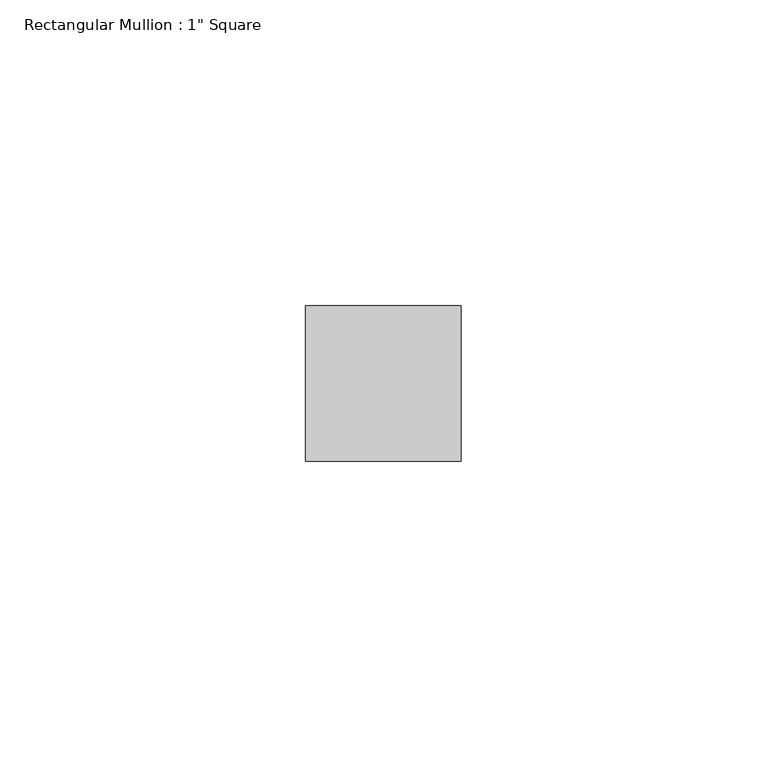
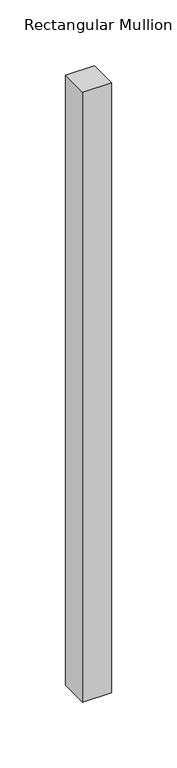
"""IFC4 building model written with IfcOpenShell, lengths in millimetres: member geometry."""

from ifc_helpers import new_model, si_unit, frame, origin, place, context, project, spatial, polyline, outline, extrude, source, transform, mapped, element, save


def member_31f2b2ad(model_context):
    return source(origin(), model_context, "Body", "SweptSolid", [
        extrude(outline(polyline([(0.0, 12.7), (0.0, -12.7), (-25.4, -12.7), (-25.4, 12.7), (0.0, 12.7)])), frame((0.0, 0.0, -565.15), z_axis=(0.0, 0.0, 1.0), x_axis=(1.0, 0.0, 0.0)), (0.0, 0.0, 1.0), 565.15),
    ])


if __name__ == "__main__":
    model = new_model("IFC4")
    model_context = context("Model", 3, world=origin())
    ifc_project = project(units=[si_unit("LENGTHUNIT", "METRE", prefix="MILLI")], contexts=[model_context])
    site = spatial("IfcSite", under=ifc_project)
    building = spatial("IfcBuilding", under=site)
    placement = place(None, origin())
    member_shape = member_31f2b2ad(model_context)
    element("IfcMember", 1, ObjectType="Rectangular Mullion : 1\" Square", at=placement, inside=building, context=model_context, shape_type="MappedRepresentation", body=[
        mapped(member_shape, transform((0.0, 0.0, 0.0), x_axis=(1.0, 0.0, 0.0), y_axis=(0.0, 1.0, 0.0), z_axis=(0.0, 0.0, 1.0))),
    ])
    save(model, "model.ifc")

# Revit data of these elements
# Type "Rectangular Mullion : 1\" Square"
#   built-in parameter 1007304 = 0.0833333 (stored number, unit not read)
#   built-in parameter 1007301 = 0.0416667 (stored number, unit not read)
#   built-in parameter 1007300 = 0.0416667 (stored number, unit not read)
